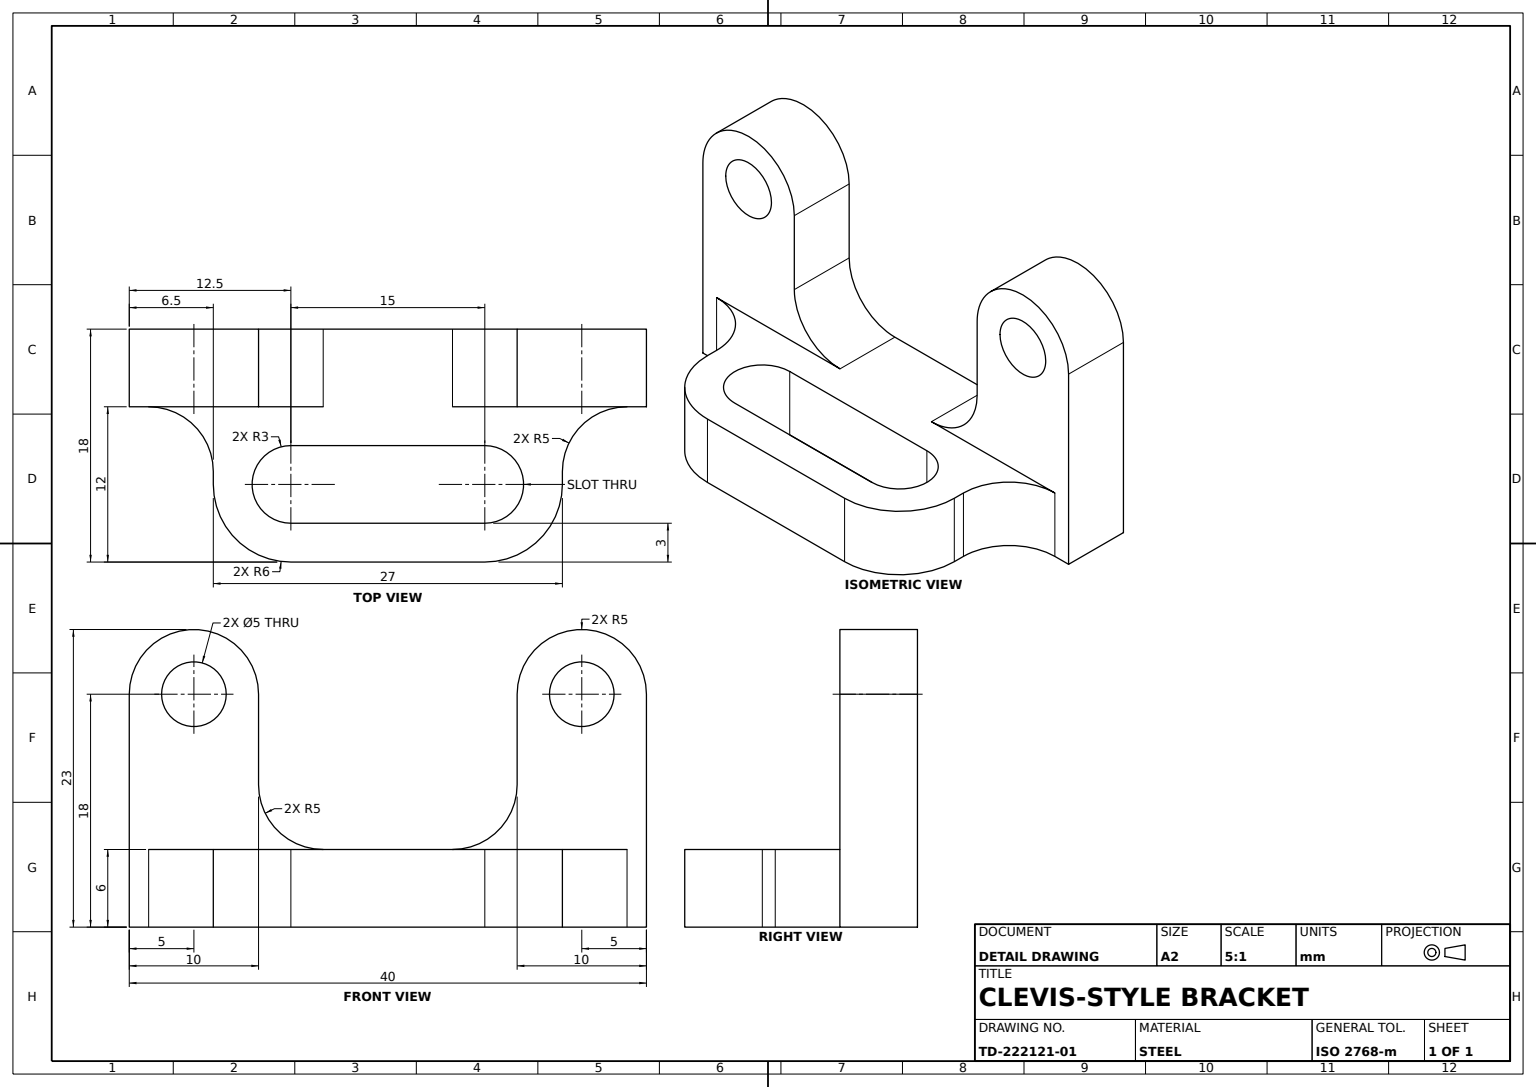
SolidWorks part; units mm, degrees
material "Plain Carbon Steel"
ref_plane "Front Plane" through (0, 0, 0) normal (0, 0, 1) x (1, 0, 0)
ref_plane "Top Plane" through (0, 0, 0) normal (0, 1, 0) x (1, 0, 0)
ref_plane "Right Plane" through (0, 0, 0) normal (1, 0, 0) x (0, 0, -1)
sketch "Bracket Profile Sketch" plane through (0, 0, 0) normal (0, 0, 1) x (1, 0, 0)
  line L0 (-20, 0) -> (20, 0)
  line L1 (-20, 0) -> (-20, 18)
  line L2 (20, 0) -> (20, 18)
  line L3 (-20, 18) -> (-15, 18)
  line L4 (20, 18) -> (15, 18)
  line L5 (-10, 18) -> (-10, 6)
  line L6 (-10, 6) -> (10, 6)
  line L7 (10, 6) -> (10, 18)
  arc A0 (-10, 18) -> (-20, 18) centre (-15, 18) ccw
  arc A1 (20, 18) -> (10, 18) centre (15, 18) ccw
  point P4 (0, 0)
  dimension "D4" = 18
  dimension "D1" = 40
  dimension "D2" = 5
  dimension "D3" = 5
  dimension "D5" = 18
  dimension "D6" = 6
extrude "Bracket Profile" add sketch "Bracket Profile Sketch" along normal blind 6
fillet "Upright Rounds R5" radius 5 2 edges at (10, 6, 3) (-10, 6, 3)
sketch "Base Plate Sketch" plane through (0, 0, 6) normal (0, 0, 1) x (1, 0, 0)
  line L0 (-20, 0) -> (20, 0) construction
  line L1 (-13.5, 0) -> (13.5, 0)
  line L2 (-13.5, 0) -> (-13.5, 6)
  line L3 (-13.5, 6) -> (13.5, 6)
  line L4 (13.5, 0) -> (13.5, 6)
  dimension "D1" = 27
  dimension "D2" = 13.5
  dimension "D3" = 6
extrude "Base Plate" add sketch "Base Plate Sketch" along normal blind 12
fillet "Base Plate Rounds R6" radius 6 2 edges at (-13.5, 3, 18) (13.5, 3, 18)
fillet "Base-Upright Fillets R5" radius 5 2 edges at (13.5, 3, 6) (-13.5, 3, 6)
sketch "Base Slot Sketch" plane through (0, 6, 0) normal (0, 1, 0) x (1, 0, 0)
  line L0 (-7.5, -12) -> (7.5, -12) construction
  line L1 (-7.5, -9) -> (7.5, -9)
  line L2 (-7.5, -15) -> (7.5, -15)
  arc A0 (-7.5, -9) -> (-7.5, -15) centre (-7.5, -12) ccw
  arc A1 (7.5, -15) -> (7.5, -9) centre (7.5, -12) ccw
  point P4 (0, -12)
  dimension "D1" = 3
extrude "Base Slot" cut sketch "Base Slot Sketch" against normal blind 6
sketch "Pivot Holes Sketch" plane through (0, 0, 6) normal (0, 0, 1) x (1, 0, 0)
  circle A0 centre (-15, 18) radius 2.5
  circle A1 centre (15, 18) radius 2.5
  dimension "D1" = 5
  dimension "D2" = 5
extrude "Pivot Holes 2xØ5" cut sketch "Pivot Holes Sketch" against normal blind 6
